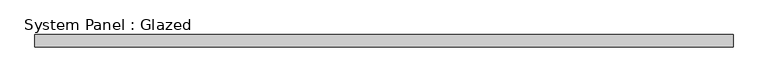
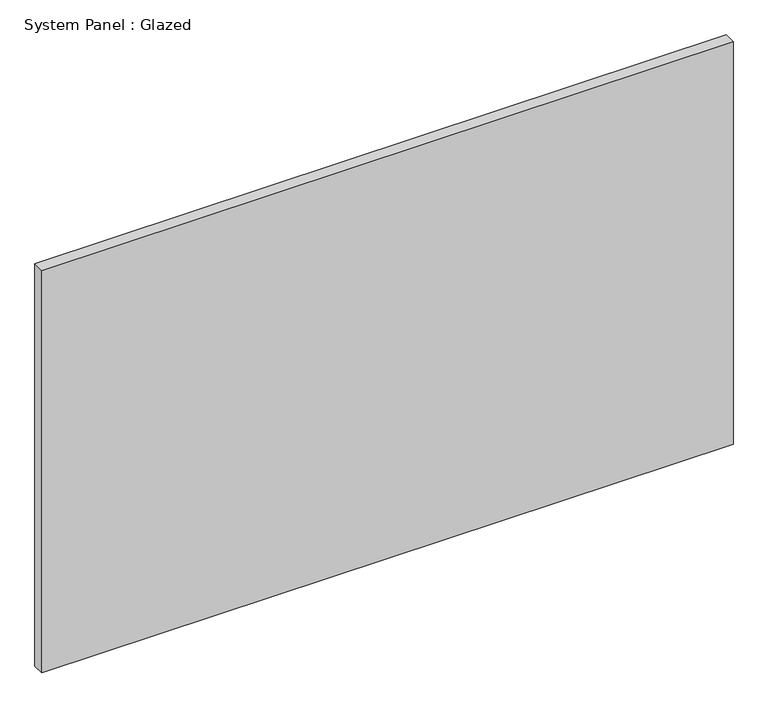
"""IFC4 building model written with IfcOpenShell, lengths in millimetres: plate geometry, System Panel : Glazed."""

from ifc_helpers import new_model, si_unit, origin, origin_with_axes, place, context, project, spatial, polyline, outline, extrude, source, transform, mapped, element, save


def system_panel_glazed_8bce9487(model_context):
    return source(origin(), model_context, "Body", "SweptSolid", [
        extrude(outline(polyline([(729.1876831, 19.05), (-729.1876831, 19.05), (-729.1876831, 44.45), (729.1876831, 44.45), (729.1876831, 19.05)])), origin_with_axes(), (0.0, 0.0, 1.0), 897.3037122),
    ])


if __name__ == "__main__":
    model = new_model("IFC4")
    model_context = context("Model", 3, world=origin())
    ifc_project = project(units=[si_unit("LENGTHUNIT", "METRE", prefix="MILLI")], contexts=[model_context])
    site = spatial("IfcSite", under=ifc_project)
    building = spatial("IfcBuilding", under=site)
    placement = place(None, origin())
    system_panel_glazed_shape = system_panel_glazed_8bce9487(model_context)
    element("IfcPlate", 1, ObjectType="System Panel : Glazed", at=placement, inside=building, context=model_context, shape_type="MappedRepresentation", body=[
        mapped(system_panel_glazed_shape, transform((0.0, 0.0, 0.0), x_axis=(1.0, 0.0, 0.0), y_axis=(0.0, 1.0, 0.0), z_axis=(0.0, 0.0, 1.0))),
    ])
    save(model, "model.ifc")

# Revit data of these elements
# Type "System Panel : Glazed"
#   Construction Type Id = "GSP4R"
#   Analytic Construction = "1/8 in Pilkington single glazing"
#   Visual Light Transmittance = 0.9
#   Solar Heat Gain Coefficient = 0.86
#   Heat Transfer Coefficient (U) = 1.18115 BTU/(h·ft²·°F)
#   Define Thermal Properties by = 1
# Element 1 (IfcPlate, "System Panel : Glazed")
#   Materials on its faces: "Glass"
# Materials
#   "Glass": class "Glass", colour RGB 0 128 192, transparency 0.75, Description = "Soda Lime Glass", Cost = 0
